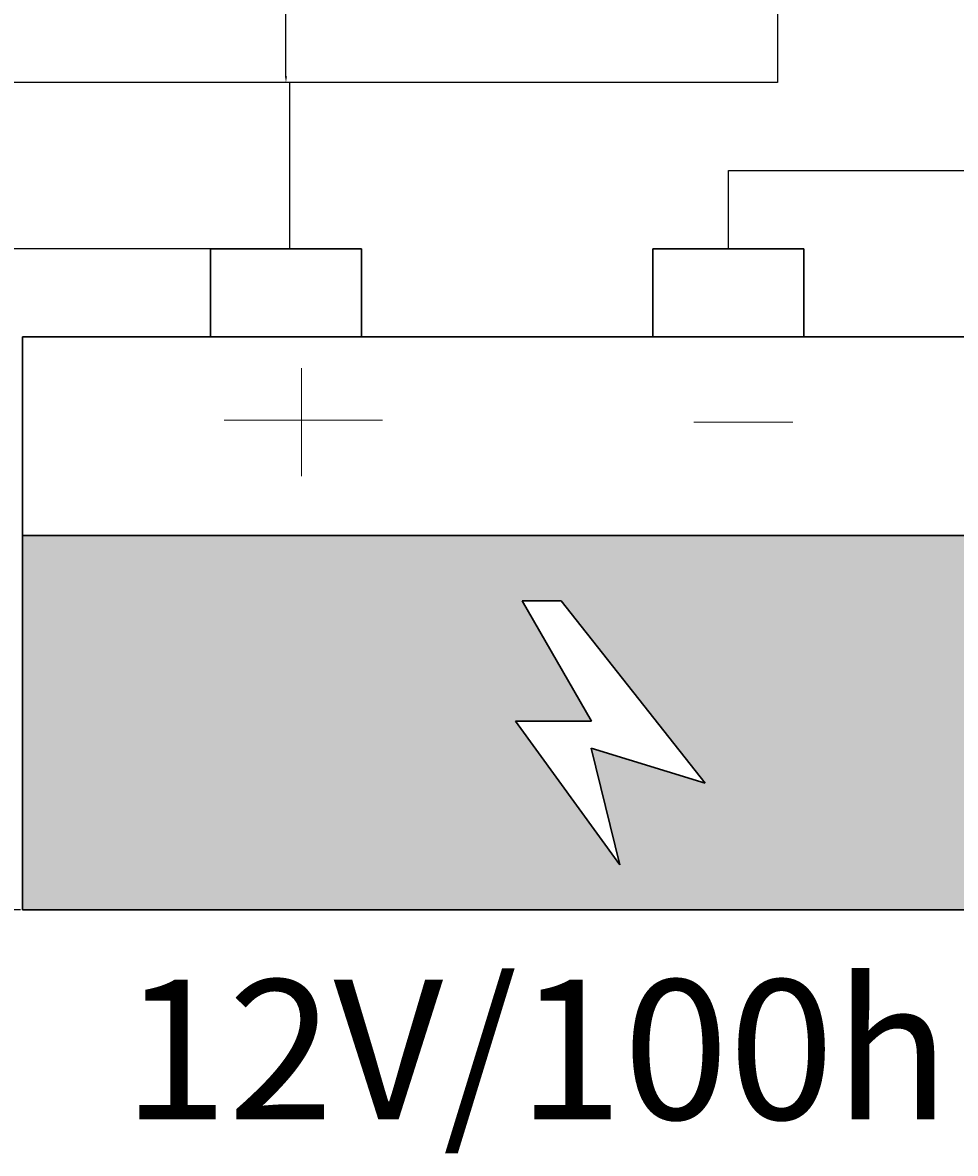
# Model space of a CAD drawing. Units: millimetres. Extents: x -8 to 285, y 5 to 221.
# Tile 2 of 30: x 31 to 57, y 13 to 45. Entities that reach past the tile are written whole.
import ezdxf

# ---------------------------------------------------------------- set-up
doc = ezdxf.new("R2010")
doc.units = ezdxf.units.MM
for name, color, linetype, lineweight in [('A-ANNO-DIMS', 2, 'Continuous', 18), ('E-ANNO-SYMB', 7, 'Continuous', 18), ('E-ANNO-TEXT', 7, 'Continuous', 18), ('E-EQPM-PATT', 252, 'Continuous', 13), ('E-POWR-BATT', 7, 'Continuous', 30), ('E-POWR-DC-LINK', 4, 'Continuous', 25)]:
    doc.layers.add(name, color=color, linetype=linetype, lineweight=lineweight)
doc.layers.add('E-POWR-DC-POS', color=30, linetype='Continuous', lineweight=25, true_color=0xf26722)
doc.styles.get("Standard").update_dxf_attribs({"font": 'arial.ttf'})
doc.dimstyles.get("Standard").update_dxf_attribs({"dimtxt": 0.18, "dimasz": 0.18, "dimexe": 0.18, "dimexo": 0.0625, "dimgap": 0.09, "dimtad": 0, "dimtih": 1, "dimtoh": 1, "dimdec": 4, "dimzin": 0, "dimdsep": 46, "dimtxsty": 'Standard', "dimcen": 0.09, "dimadec": 0, "dimazin": 0, "dimtfac": 1, "dimtdec": 4, "dimtofl": 0, "dimtmove": 0, "dimatfit": 3, "dimfxl": 1, "dimtolj": 1, "dimtzin": 0, "dimarcsym": 0})

# ---------------------------------------------------------------- blocks, each defined once
blk = doc.blocks.new('BATTERY-CASE')
blk.add_line((0, 10.738), (31.163, 10.738))
blk.add_lwpolyline([(0, 16.427), (31.163, 16.427), (31.163, 0), (0, 0)], close=True)
blk = doc.blocks.new('BATTERY-TERMINAL-POST')
for p, q in [((0, 0), (0, 2.525)), ((0, 2.525), (4.334, 2.525)), ((4.334, 2.525), (4.334, 0))]:
    blk.add_line(p, q)
blk = doc.blocks.new('BATTERY-LIGHTNING-EMBLEM')
for p, q in [((2.173, 4.126), (0.184, 7.57)), ((0.184, 7.57), (1.304, 7.57)), ((5.441, 2.343), (1.304, 7.57)), ((0, 4.126), (2.173, 4.126)), ((2.991, 0), (0, 4.126)), ((5.441, 2.343), (2.169, 3.351)), ((2.169, 3.351), (2.991, 0))]:
    blk.add_line(p, q)
blk = doc.blocks.new('POLARITY-POSITIVE')
for p, q in [((2.22, 3.095), (2.22, 0)), ((0, 1.599), (4.543, 1.599))]:
    blk.add_line(p, q)
blk = doc.blocks.new('*D10')
at = {"layer": 'A-ANNO-DIMS', "color": 0, "lineweight": -2, "transparency": 16777216}
for p, q in [((145.103, 206.457), (-7.608, 206.457)), ((-7.428, 206.277), (-7.428, 113.161)), ((-7.428, 19.682), (-7.428, 112.797)), ((30.453, 19.502), (-7.608, 19.502))]:
    blk.add_line(p, q, dxfattribs=at)
at = {"layer": 'A-ANNO-DIMS', "color": 0, "transparency": 16777216}
for points in [[(-7.458, 206.277), (-7.398, 206.277), (-7.428, 206.457)], [(-7.458, 19.682), (-7.398, 19.682), (-7.428, 19.502)]]:
    blk.add_solid(points, dxfattribs=at)
at = {"layer": 'Defpoints', "color": 0, "transparency": 16777216}
for p in [(-7.428, 206.457), (145.165, 206.457), (30.516, 19.502)]:
    blk.add_point(p, dxfattribs=at)
at = {"layer": 'A-ANNO-DIMS', "color": 0, "transparency": 16777216, "insert": (-7.428, 112.979), "char_height": 0.18, "attachment_point": 5}
blk.add_mtext('\\A1;186.95', dxfattribs=at)
blk = doc.blocks.new('*D20')
at = {"layer": 'A-ANNO-DIMS', "color": 0, "lineweight": -2, "transparency": 16777216}
for p, q in [((38.112044, 43.223892), (23.894544, 43.223892)), ((24.074544, 43.043892), (24.074544, 41.018795)), ((24.074544, 38.633698), (24.074544, 40.658795)), ((38.112044, 38.453698), (23.894544, 38.453698))]:
    blk.add_line(p, q, dxfattribs=at)
at = {"layer": 'A-ANNO-DIMS', "color": 0, "transparency": 16777216}
for points in [[(24.044544, 43.043892), (24.104544, 43.043892), (24.074544, 43.223892)], [(24.044544, 38.633698), (24.104544, 38.633698), (24.074544, 38.453698)]]:
    blk.add_solid(points, dxfattribs=at)
at = {"layer": 'Defpoints', "color": 0, "transparency": 16777216}
for p in [(24.074544, 43.223892), (38.174544, 43.223892), (38.174544, 38.453698)]:
    blk.add_point(p, dxfattribs=at)
at = {"layer": 'A-ANNO-DIMS', "color": 0, "transparency": 16777216, "insert": (24.074544, 40.838795), "char_height": 0.18, "attachment_point": 5}
blk.add_mtext('\\A1;4.77', dxfattribs=at)
blk = doc.blocks.new('*D21')
at = {"layer": 'A-ANNO-DIMS', "color": 0, "lineweight": -2, "transparency": 16777216}
for p, q in [((52.109, 67.906), (37.892, 67.906)), ((38.072, 67.726), (38.072, 55.747)), ((38.072, 43.404), (38.072, 55.383)), ((52.109, 43.224), (37.892, 43.224))]:
    blk.add_line(p, q, dxfattribs=at)
at = {"layer": 'A-ANNO-DIMS', "color": 0, "transparency": 16777216}
for points in [[(38.042, 67.726), (38.102, 67.726), (38.072, 67.906)], [(38.042, 43.404), (38.102, 43.404), (38.072, 43.224)]]:
    blk.add_solid(points, dxfattribs=at)
at = {"layer": 'Defpoints', "color": 0, "transparency": 16777216}
for p in [(38.072, 67.906), (52.172, 67.906), (52.172, 43.224)]:
    blk.add_point(p, dxfattribs=at)
at = {"layer": 'A-ANNO-DIMS', "color": 0, "transparency": 16777216, "insert": (38.072, 55.565), "char_height": 0.18, "attachment_point": 5}
blk.add_mtext('\\A1;24.683', dxfattribs=at)

msp = doc.modelspace()

# ---------------------------------------------------------------- hatches: boundary and pattern name
at = {"layer": 'E-EQPM-PATT'}
h = msp.add_hatch(color=256, dxfattribs=at)
h.set_gradient(color1=(244, 238, 81), color2=(248, 153, 30), tint=1)
h.paths.add_polyline_path([(30.516, 30.2396), (30.516, 19.502), (61.6786, 19.502), (61.6786, 30.2396)])
h.paths.add_polyline_path([(44.6613, 24.9143), (46.8335, 24.9143), (44.845, 28.3584), (45.9646, 28.3584), (50.1024, 23.1306), (46.8299, 24.1393), (47.652, 20.7882)], flags=16)
h.paths.add_polyline_path([(72.6568, 30.2396), (72.6568, 19.502), (103.8194, 19.502), (103.8194, 30.2396)])
h.paths.add_polyline_path([(86.2008, 24.9143), (88.373, 24.9143), (86.3846, 28.3584), (87.5041, 28.3584), (91.6419, 23.1306), (88.3694, 24.1393), (89.1915, 20.7882)], flags=16)

# ---------------------------------------------------------------- linework, layer by layer
at = {"layer": 'E-ANNO-SYMB'}
msp.add_line((49.7738, 33.4874), (52.6133, 33.4874), dxfattribs=at)
at = {"layer": 'E-POWR-DC-LINK'}
msp.add_line((50.7659, 38.4537), (50.7659, 40.7074), dxfattribs=at)
msp.add_lwpolyline([(50.7659, 40.7074), (80.3875, 40.7074), (80.3759, 38.4537)], dxfattribs=at)
at = {"layer": 'E-POWR-DC-POS'}
msp.add_lwpolyline([(52.1717, 67.9064), (52.1717, 43.2239), (38.1745, 43.2239), (38.1745, 38.4537)], dxfattribs=at)

# ---------------------------------------------------------------- block references
at = {"layer": 'E-ANNO-SYMB'}
msp.add_blockref('POLARITY-POSITIVE', (36.299, 31.94), dxfattribs=at)
at = {"layer": 'E-POWR-BATT'}
for name, p in [('BATTERY-TERMINAL-POST', (35.909, 35.929)), ('BATTERY-TERMINAL-POST', (48.599, 35.929)), ('BATTERY-CASE', (30.516, 19.502)), ('BATTERY-LIGHTNING-EMBLEM', (44.661, 20.788))]:
    msp.add_blockref(name, p, dxfattribs=at)

# ---------------------------------------------------------------- texts
at = {"layer": 'E-ANNO-TEXT', "insert": (33.3813, 17.4943), "char_height": 4, "attachment_point": 1}
msp.add_mtext_dynamic_manual_height_columns('12V/100h            12V/100Ah', width=74.08228, gutter_width=12.5, heights=[0], dxfattribs=at)

# ---------------------------------------------------------------- dimensions: what is measured, and where the dimension line sits
at = {"layer": 'A-ANNO-DIMS'}
for base, p1, p2, override, picture, middle in [((-7.4275, 206.4568), (30.516, 19.502), (145.1651, 206.4568), {"dimdec": 2, "dimlfac": 1, "dimrnd": 0, "dimzin": 0, "dimdsep": 46, "dimlunit": 2}, '*D10', (-7.4275, 112.9794)), ((38.07166, 67.90641), (52.17166, 43.22389), (52.17166, 67.90641), {"dimdec": 3, "dimlfac": 1, "dimrnd": 0, "dimzin": 0, "dimdsep": 46, "dimlunit": 2}, '*D21', (38.07166, 55.56515)), ((24.0745, 43.2239), (38.1745, 38.4537), (38.1745, 43.2239), {"dimdec": 2, "dimlfac": 1, "dimrnd": 0, "dimzin": 0, "dimdsep": 46, "dimlunit": 2}, '*D20', (24.0745, 40.8388))]:
    dim = msp.add_linear_dim(base=base, p1=p1, p2=p2, angle=90, dimstyle='Standard', override=override, dxfattribs=at)
    dim.commit()
    dim.dimension.update_dxf_attribs({"geometry": picture, "text_midpoint": middle})

doc.saveas('drawing.dxf')
